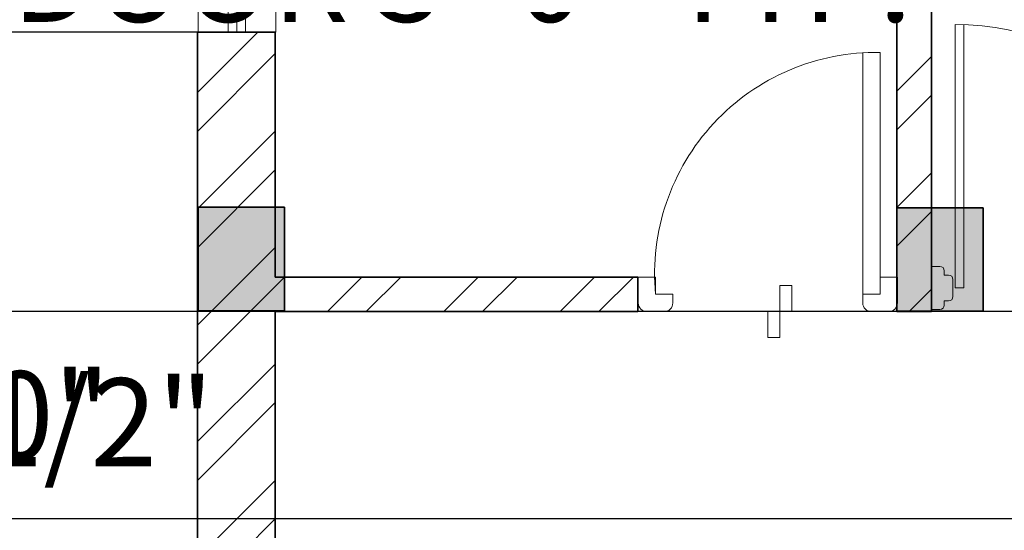
# Model space of a CAD drawing. Units: inches. Extents: x 1812 to 2791, y 2306 to 2959.
# Tile 3 of 8: x 1870 to 1984, y 2715 to 2774. Entities that reach past the tile are written whole.
import ezdxf

# ---------------------------------------------------------------- set-up
doc = ezdxf.new("R2010")
doc.units = ezdxf.units.IN
doc.linetypes.add('ACAD_ISO02W100', pattern=[15, 12, -3])
doc.layers.get('Defpoints').update_dxf_attribs({"lineweight": 50})
for name, color, linetype, lineweight in [('00 FURNITURE', 15, 'Continuous', 15), ('A-ANNO-DIMS', 2, 'Continuous', 18), ('A-COLS', 7, 'Continuous', 35), ('A-GLAZ-VENT', 6, 'ACAD_ISO02W100', 13), ('A-WALL-PATT', 8, 'Continuous', 13), ('A_FUR 1', 5, 'Continuous', 5), ('DOORS', 4, 'Continuous', 18), ('WALL', 7, 'Continuous', 35)]:
    doc.layers.add(name, color=color, linetype=linetype, lineweight=lineweight)
doc.styles.get("Standard").update_dxf_attribs({"font": 'arial.ttf'})
doc.dimstyles.get("Standard").update_dxf_attribs({"dimtxt": 10.18, "dimasz": 0.18, "dimexe": 0.18, "dimexo": 0.0625, "dimgap": 0.09, "dimtad": 0, "dimtih": 1, "dimtoh": 1, "dimdec": 0, "dimzin": 0, "dimdsep": 46, "dimlunit": 3, "dimtxsty": 'Standard', "dimcen": 0.09, "dimadec": 0, "dimazin": 0, "dimtfac": 1, "dimtdec": 0, "dimtofl": 0, "dimtmove": 0, "dimatfit": 3, "dimfxl": 1, "dimtolj": 1, "dimtzin": 0, "dimarcsym": 0})

# ---------------------------------------------------------------- blocks, each defined once
blk = doc.blocks.new('ESTSET')
at = {"layer": 'A_FUR 1'}
for p, q in [((-10.44359699611232, 4.096573562603225), (-10.44359699611232, 32.09657356260323)), ((-8.44359699611232, 4.096573562603225), (-8.44359699611232, 32.09657356260323)), ((-36.44359699611232, 6.096573562603225), (-36.44359699611232, 3.096573562603225)), ((-34.44359699611232, 6.096573562603225), (-36.44359699611232, 6.096573562603225)), ((-34.44359699611232, 4.096573562603225), (-34.44359699611232, 6.096573562603225)), ((-34.44359699611232, 4.096573562603225), (-34.44359699611232, 6.096573562603225)), ((-8.44359699611232, 4.096573562603225), (-8.44359699611232, 6.096573562603225)), ((-8.44359699611232, 6.096573562603225), (-6.443596996112319, 6.096573562603225)), ((-8.44359699611232, 4.096573562603225), (-8.44359699611232, 6.096573562603225)), ((-6.443596996112319, 6.096573562603225), (-6.443596996112319, 3.096573562603225)), ((-32.44359699611232, 4.096573562603225), (-34.44359699611232, 4.096573562603225)), ((-32.44359699611232, 4.096573562603225), (-34.44359699611232, 4.096573562603225)), ((-32.44359699611232, 3.096573562603225), (-32.44359699611232, 4.096573562603225)), ((-10.44359699611232, 3.096573562603225), (-10.44359699611232, 4.096573562603225)), ((-10.44359699611232, 4.096573562603225), (-8.44359699611232, 4.096573562603225)), ((-10.44359699611232, 4.096573562603225), (-8.44359699611232, 4.096573562603225)), ((-6.443596996112319, 2.096573562601521), (-36.4435969961196, 2.09657356260334)), ((-35.44359699611232, 2.096573562603225), (-33.44359699611232, 2.096573562603225)), ((-7.443596996112319, 2.096573562603225), (-9.44359699611232, 2.096573562603225))]:
    blk.add_line(p, q, dxfattribs=at)
for points in [[(-21.44359699614506, 2.09657356260334), (-18.67227073841423, 2.09657356260334), (-18.67227073841423, 5.101808480258228), (-20.05793386727964, 5.101808480258228)], [(-20.05793386727964, 5.101808480258228), (-20.05793386727964, -0.9086613550515485)], [(-21.44359699614506, 2.09657356260334), (-21.44359699614506, -0.9086613550515485), (-20.05793386727964, -0.9086613550515485)]]:
    blk.add_lwpolyline(points, dxfattribs=at)
for centre, radius, start, end in [((-8.908777800232201, 6.457098594999479), 25.64369454261379, 88.96058819788949, 185.2816045955121), ((-35.44359699611232, 3.096573562603225), 1, 180, 270), ((-33.44359699611232, 3.096573562603225), 1, 270, 0), ((-9.44359699611232, 3.096573562603225), 1, 180, 270), ((-7.443596996112319, 3.096573562603225), 1, 270, 0)]:
    blk.add_arc(centre, radius, start, end, dxfattribs=at)
blk = doc.blocks.new('DDD')
at = {"layer": '00 FURNITURE'}
for p, q in [((-12579.77346126611, -15859.52901419652), (-12579.77346126608, -15829.04541204713)), ((-12578.77346126611, -15859.52901419657), (-12578.77346126608, -15829.02901419657)), ((-12612.02346126613, -15857.02901419646), (-12612.02346126613, -15862.02901419646)), ((-12611.02346126613, -15857.02901419646), (-12612.02346126613, -15857.02901419646)), ((-12610.52346126612, -15858.02901419646), (-12610.52346126612, -15857.52901419646)), ((-12577.52346126611, -15858.02901419658), (-12577.52346126611, -15857.52901419657)), ((-12577.02346126611, -15857.02901419657), (-12576.02346126611, -15857.02901419652)), ((-12576.02346126611, -15857.02901419652), (-12576.02346126611, -15862.02901419652)), ((-12578.77346126611, -15859.52901419657), (-12579.77346126611, -15859.52901419652)), ((-12610.52346126612, -15861.52901419646), (-12610.52346126612, -15861.02901419646)), ((-12577.52346126611, -15861.52901419657), (-12577.52346126611, -15861.02901419657)), ((-12612.02346126613, -15862.02901419646), (-12611.02346126613, -15862.02901419646)), ((-12576.02346126611, -15862.02901419652), (-12577.02346126611, -15862.02901419657))]:
    blk.add_line(p, q, dxfattribs=at)
for points in [[(-12610.52346126612, -15861.02901419646), (-12610.02346126613, -15861.02901419646, 0.4142135623730951), (-12609.52346126612, -15860.52901419646), (-12609.52346126612, -15858.52901419646, 0.4142135623730951), (-12610.02346126613, -15858.02901419646), (-12610.52346126612, -15858.02901419646)], [(-12577.52346126611, -15861.02901419657), (-12578.02346126611, -15861.02901419657, -0.4142135623730951), (-12578.52346126611, -15860.52901419657), (-12578.52346126611, -15858.52901419657, -0.4142135623730951), (-12578.02346126611, -15858.02901419658), (-12577.52346126611, -15858.02901419658)]]:
    blk.add_lwpolyline(points, format="xyb", dxfattribs=at)
for centre, radius, start, end in [((-12578.77346126613, -15859.52901419657), 30.49999999999949, 90, 180), ((-12611.02346126613, -15857.52901419646), 0.4999999999999916, 0, 90), ((-12577.02346126611, -15857.52901419657), 0.4999999999999916, 90, 180), ((-12611.02346126613, -15861.52901419646), 0.4999999999999916, 270, 0), ((-12577.02346126611, -15861.52901419657), 0.4999999999999916, 180, 270)]:
    blk.add_arc(centre, radius, start, end, dxfattribs=at)
blk = doc.blocks.new('COL')
at = {"transparency": 33554687}
h = blk.add_hatch(color=256, dxfattribs=at)
h.dxf.hatch_style = 1
h.paths.add_polyline_path([(2424.397880689844, 2829.240948453883), (2424.397880689844, 2839.240948453883), (2412.397880689843, 2839.240948453883), (2412.397880689843, 2829.240948453883)])
for p, q in [((2412.397880689843, 2839.240948453883), (2424.397880689844, 2839.240948453883)), ((2412.397880689843, 2839.240948453883), (2412.397880689843, 2829.240948453882)), ((2424.397880689844, 2839.240948453883), (2424.397880689844, 2829.240948453883)), ((2412.397880689843, 2829.240948453883), (2424.397880689844, 2829.240948453883))]:
    blk.add_line(p, q)
blk = doc.blocks.new('VENT-24x9')
for p, q in [((3.499863851171994, 23.99973038050894), (3.499863851171994, -0.0002696194910641)), ((4.499863851171994, 23.99973038050894), (4.499863851171994, -0.0002696194910641)), ((5.499863851171994, 23.99973038050894), (5.499863851171994, -0.0002696194910641))]:
    blk.add_line(p, q)
blk.add_lwpolyline([(-0.0001361485951747, -0.0002696194910641), (8.999863851404825, -0.0002696194910641), (8.999863851171995, 23.99973038050894), (-0.0001361488280054, 23.99973038050894)], close=True)
blk = doc.blocks.new('*D42')
at = {"layer": 'A-ANNO-DIMS', "color": 0, "lineweight": -2, "transparency": 16777216}
for p, q in [((1975.370579728209, 2779.236987448721), (1975.190579728209, 2779.236987448721)), ((1975.370579728209, 2773.899487448718), (1975.370579728209, 2779.416987448721)), ((2011.190579728229, 2779.236987448721), (1975.550579728209, 2779.236987448721)), ((2011.370579728229, 2773.899487448718), (2011.370579728229, 2779.416987448721))]:
    blk.add_line(p, q, dxfattribs=at)
at = {"layer": 'A-ANNO-DIMS', "color": 0, "transparency": 16777216}
for points in [[(1975.550579728209, 2779.266987448721), (1975.550579728209, 2779.206987448721), (1975.370579728209, 2779.236987448721)], [(2011.190579728229, 2779.266987448721), (2011.190579728229, 2779.206987448721), (2011.370579728229, 2779.236987448721)]]:
    blk.add_solid(points, dxfattribs=at)
at = {"layer": 'Defpoints', "color": 0, "transparency": 16777216}
for p in [(1975.370579728209, 2779.236987448721), (1975.370579728209, 2773.836987448718), (2011.370579728229, 2773.836987448718)]:
    blk.add_point(p, dxfattribs=at)
at = {"layer": 'A-ANNO-DIMS', "color": 0, "transparency": 16777216, "insert": (1921.020197736394, 2779.236987448721), "char_height": 10.18, "attachment_point": 5}
blk.add_mtext('\\A1;DOOR 3\'-0" TYP.', dxfattribs=at)
blk = doc.blocks.new('*D78')
at = {"layer": 'A-ANNO-DIMS', "color": 0, "lineweight": -2, "transparency": 16777216}
for p, q in [((1890.395003000001, 2772.947203000001), (1864.780736000002, 2772.947203000001)), ((1864.960736000002, 2772.767203000001), (1864.960736000002, 2733.146461637109)), ((1864.960736000002, 2682.818517000001), (1864.960736000002, 2722.439258362893)), ((1890.148236000001, 2682.638517000001), (1864.780736000002, 2682.638517000001))]:
    blk.add_line(p, q, dxfattribs=at)
at = {"layer": 'A-ANNO-DIMS', "color": 0, "transparency": 16777216}
for points in [[(1864.930736000002, 2772.767203000001), (1864.990736000002, 2772.767203000001), (1864.960736000002, 2772.947203000001)], [(1864.930736000002, 2682.818517000001), (1864.990736000002, 2682.818517000001), (1864.960736000002, 2682.638517000001)]]:
    blk.add_solid(points, dxfattribs=at)
at = {"layer": 'Defpoints', "color": 0, "transparency": 16777216}
for p in [(1890.457503000001, 2772.947203000001), (1864.960736000002, 2682.638517000001), (1890.210736000001, 2682.638517000001)]:
    blk.add_point(p, dxfattribs=at)
at = {"layer": 'A-ANNO-DIMS', "color": 0, "transparency": 16777216, "insert": (1864.960736000002, 2727.79286), "char_height": 10.18, "attachment_point": 5}
blk.add_mtext('\\A1;7\'-6 1/2"', dxfattribs=at)
blk = doc.blocks.new('*D81')
at = {"layer": 'A-ANNO-DIMS', "color": 0, "lineweight": -2, "transparency": 16777216}
for p, q in [((2011.324042000001, 2740.602944000001), (1864.780736000002, 2740.602944000001)), ((1864.960736000002, 2740.422944000001), (1864.960736000002, 2733.890577015008)), ((1864.960736000002, 2716.782944000001), (1864.960736000002, 2723.315310984994)), ((2011.324042000001, 2716.602944000002), (1864.780736000002, 2716.602944000002))]:
    blk.add_line(p, q, dxfattribs=at)
at = {"layer": 'A-ANNO-DIMS', "color": 0, "transparency": 16777216}
for points in [[(1864.930736000002, 2740.422944000001), (1864.990736000002, 2740.422944000001), (1864.960736000002, 2740.602944000001)], [(1864.930736000002, 2716.782944000001), (1864.990736000002, 2716.782944000001), (1864.960736000002, 2716.602944000002)]]:
    blk.add_solid(points, dxfattribs=at)
at = {"layer": 'Defpoints', "color": 0, "transparency": 16777216}
for p in [(2011.386542000001, 2740.602944000001), (1864.960736000002, 2716.602944000002), (2011.386542000001, 2716.602944000002)]:
    blk.add_point(p, dxfattribs=at)
at = {"layer": 'A-ANNO-DIMS', "color": 0, "transparency": 16777216, "insert": (1864.960736000002, 2728.602944), "char_height": 10.18, "attachment_point": 5}
blk.add_mtext('\\A1;2\'-0"', dxfattribs=at)

msp = doc.modelspace()

# ---------------------------------------------------------------- hatches: boundary and pattern name
at = {"layer": 'A-WALL-PATT'}
h = msp.add_hatch(dxfattribs=at)
h.set_pattern_fill('ANSI32', color=256)
h.set_pattern_definition([(45, (0, 0), (-6.735192090801865, 6.735192090801866), []), (45, (4.49013, 0), (-6.735192090801865, 6.735192090801866), [])])
h.paths.add_polyline_path([(2130.386541883867, 2417.602943720933), (2119.693765675914, 2417.602943720932), (2119.693765675914, 2768.55867658318), (2121.386541883867, 2768.55867658318), (2121.386541883867, 2801.624379255592), (2121.320110177716, 2849.363725604599), (2121.320110177716, 2801.624379255592), (2130.386541883867, 2801.624379255592)])
h.paths.add_polyline_path([(2023.386541883867, 2426.602943720928), (1899.386541883867, 2426.602943720922), (1899.386541883867, 2453.602943720933), (1951.802463468582, 2453.602943720933), (1951.802463468583, 2457.602943720932), (1899.386541883867, 2457.602943720932), (1899.386541883867, 2590.602943720933), (1959.931736449602, 2590.602943720933), (1959.931736449602, 2594.602943720933), (1899.386541883867, 2594.602943720933), (1899.386541883867, 2634.525457409657), (1890.386541883867, 2634.525457409656), (1890.386541883867, 2417.602943720933), (2023.386541883867, 2417.602943720933)])
h.paths.add_polyline_path([(2119.693765675914, 2426.602943720933), (2112.386541883867, 2426.602943720932), (2112.386541883867, 2417.602943720932), (2119.693765675914, 2417.602943720933)])
h.paths.add_polyline_path([(1899.386541883867, 2740.602943720932), (1941.386541883867, 2740.602943720932), (1941.386541883866, 2744.602943720933), (1899.386541883867, 2744.602943720932), (1899.386541883867, 2772.941372394735), (1890.386541883867, 2772.941372394735), (1890.386541883867, 2682.525457409656), (1899.210735520098, 2682.525457409656), (1899.210735520098, 2682.638517261234)])
h.paths.add_polyline_path([(1975.386541883867, 2838.602943720933), (1899.386541883867, 2838.602943720932), (1899.386541883866, 2856.334456704745), (1890.386541883867, 2856.334456704745), (1890.386541883867, 2796.94720306846), (1899.386541883867, 2796.94720306846), (1899.386541883867, 2834.602943720933), (1971.386541883867, 2834.602943720933), (1971.386541883867, 2740.602943720933), (1975.386541883867, 2740.602943720933)])
h.paths.add_polyline_path([(2119.693765675914, 2897.602943720933), (1890.386541883867, 2897.602943720933), (1890.386541883867, 2880.361730380509), (1899.386541883866, 2880.361730380509), (1899.386541883867, 2888.602943720933), (2119.693765675914, 2888.602943720933)])
h.paths.add_polyline_path([(2130.386541883867, 2897.602943720933), (2119.693765675914, 2897.602943720933), (2119.693765675914, 2888.602943720933), (2121.386541883867, 2888.602943720933), (2121.386541883867, 2849.624379255592), (2130.386541883867, 2849.624379255592)])

# ---------------------------------------------------------------- linework, layer by layer
at = {"layer": 'WALL'}
for p, q in [((1975.386541883867, 2740.602943720933), (1975.386541883867, 2838.602943720932)), ((1971.386541883867, 2740.602943720933), (1971.386541883867, 2834.602943720933)), ((1890.386541883867, 2682.525457409657), (1890.386541883867, 2772.941372394735)), ((1899.386541883867, 2772.941372394735), (1890.386541883867, 2772.941372394735)), ((1899.386541883867, 2744.602943720932), (1899.386541883867, 2772.941372394735)), ((1899.386541883868, 2744.602943720932), (1941.386541883867, 2744.602943720933)), ((1941.386541883867, 2740.602943720933), (1941.386541883866, 2744.602943720933)), ((1899.386541883868, 2740.602943720932), (1941.386541883866, 2740.602943720932)), ((1899.386541883867, 2682.525457409656), (1899.386541883867, 2740.602943720932)), ((1971.386541883867, 2740.602943720933), (1975.386541883867, 2740.602943720933))]:
    msp.add_line(p, q, dxfattribs=at)

# ---------------------------------------------------------------- block references
at = {"layer": 'A-COLS', "rotation": 270}
for p in [(-938.7656370823227, 5165.081868230806), (-857.8596008978113, 5165.03255225655)]:
    msp.add_blockref('COL', p, dxfattribs=at)
at = {"layer": 'A-GLAZ-VENT'}
msp.add_blockref('VENT-24x9', (1890.45763924307, 2772.947472687951), dxfattribs=at)
at = {"layer": 'DOORS', "xscale": -1}
msp.add_blockref('DDD', (-10600.6528815379, 18602.86600164529), dxfattribs=at)
at = {"layer": 'DOORS'}
msp.add_blockref('ESTSET', (1977.878040427123, 2738.509989581549), dxfattribs=at)

# ---------------------------------------------------------------- dimensions: what is measured, and where the dimension line sits
at = {"layer": 'A-ANNO-DIMS'}
dim = msp.add_linear_dim(base=(1975.370579728209, 2779.236987448721), p1=(2011.370579728229, 2773.836987448718), p2=(1975.370579728209, 2773.836987448718), angle=180, text='DOOR <> TYP.', dimstyle='Standard', override={"dimdec": 1, "dimlfac": 1, "dimrnd": 0, "dimzin": 1, "dimdsep": 46, "dimlunit": 4, "dimfrac": 2}, dxfattribs=at)
dim.commit()
dim.dimension.update_dxf_attribs({"geometry": '*D42', "text_midpoint": (1921.020197736394, 2779.236987448721)})
for base, p1, p2, picture, middle in [((1864.960736000002, 2682.638517000001), (1890.457503, 2772.947203000001), (1890.210736, 2682.638517), '*D78', (1864.960736000002, 2727.79286)), ((1864.960736000002, 2716.602944000002), (2011.386542, 2740.602944), (2011.386542, 2716.602944), '*D81', (1864.960736000002, 2728.602944))]:
    dim = msp.add_linear_dim(base=base, p1=p1, p2=p2, angle=90, dimstyle='Standard', override={"dimdec": 1, "dimlfac": 1, "dimrnd": 0, "dimzin": 1, "dimdsep": 46, "dimlunit": 4, "dimfrac": 2}, dxfattribs=at)
    dim.commit()
    dim.dimension.update_dxf_attribs({"geometry": picture, "text_midpoint": middle})

doc.saveas('drawing.dxf')
